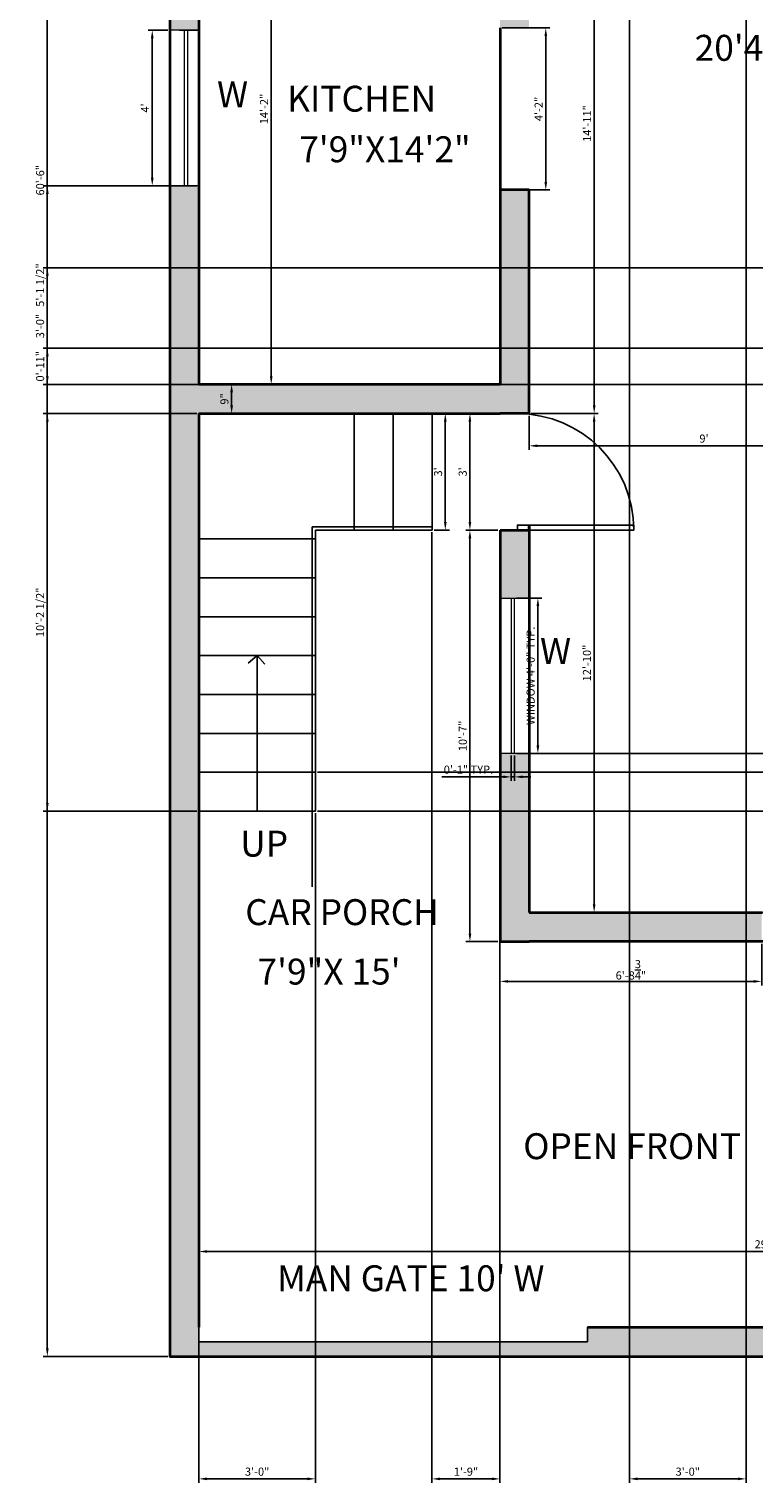
# Model space of a CAD drawing. Units: inches. Extents: x 844 to 1293, y 1224 to 2014.
# Tile 1 of 4: x 844 to 1068, y 1224 to 1673. Entities that reach past the tile are written whole.
import ezdxf

# ---------------------------------------------------------------- set-up
doc = ezdxf.new("R2010")
doc.units = ezdxf.units.IN
for name, color, linetype, lineweight in [('A-ANNO-DIMS', 2, 'Continuous', 18), ('A-ANNO-TEXT', 3, 'Continuous', 18), ('A-AREA-IDEN', 7, 'Continuous', 25), ('A-DOOR', 3, 'Continuous', 25), ('A-FLOR-STRS', 7, 'Continuous', 25), ('A-GLAZ', 4, 'Continuous', 18), ('A-WALL', 7, 'Continuous', 35), ('A-WALL-PATT', 252, 'Continuous', 13)]:
    doc.layers.add(name, color=color, linetype=linetype, lineweight=lineweight)
doc.styles.get("Standard").update_dxf_attribs({"font": 'arial.ttf'})
doc.dimstyles.new('Copy of ISO-25', dxfattribs={"dimtxt": 2.5, "dimasz": 2.5, "dimexe": 1.25, "dimexo": 0.625, "dimtad": 1, "dimlunit": 4, "dimtxsty": 'Standard', "dimcen": 2.5, "dimadec": 0, "dimazin": 0, "dimtfac": 1, "dimtmove": 0, "dimatfit": 3, "dimfxl": 1, "dimarcsym": 0})

# ---------------------------------------------------------------- blocks, each defined once
blk = doc.blocks.new('*U4')
for p, q in [((0, 0), (0, -6)), ((-40, 0), (-40, -6))]:
    blk.add_line(p, q)
blk.add_lwpolyline([(0, 0), (0, 40), (-1.75, 40), (-1.75, 0)], close=True)
blk.add_arc((0, 0), 40, 90, 180)
blk = doc.blocks.new('*D16')
at = {"layer": 'A-ANNO-DIMS', "color": 0, "lineweight": -2, "transparency": 16777216}
for p, q in [((897.09, 1733.04), (920.05, 1733.04)), ((918.8, 1730.54), (918.8, 1565.54)), ((897.09, 1563.04), (920.05, 1563.04))]:
    blk.add_line(p, q, dxfattribs=at)
at = {"layer": 'A-ANNO-DIMS', "color": 0, "transparency": 16777216}
for points in [[(918.39, 1730.54), (919.22, 1730.54), (918.8, 1733.04)], [(918.39, 1565.54), (919.22, 1565.54), (918.8, 1563.04)]]:
    blk.add_solid(points, dxfattribs=at)
at = {"layer": 'Defpoints', "color": 0, "transparency": 16777216}
for p in [(896.46, 1733.04), (896.46, 1563.04), (918.8, 1563.04)]:
    blk.add_point(p, dxfattribs=at)
at = {"layer": 'A-ANNO-DIMS', "color": 0, "transparency": 16777216, "insert": (916.92, 1648.04), "char_height": 2.5, "attachment_point": 5, "rotation": 90}
blk.add_mtext('14\'-2"', dxfattribs=at)
blk = doc.blocks.new('*D17')
at = {"layer": 'A-ANNO-DIMS', "color": 0, "lineweight": -2, "transparency": 16777216}
for p, q in [((998.46, 1553.35), (998.46, 1542.83)), ((1106.46, 1553.35), (1106.46, 1542.83)), ((1000.96, 1544.08), (1103.96, 1544.08))]:
    blk.add_line(p, q, dxfattribs=at)
at = {"layer": 'A-ANNO-DIMS', "color": 0, "transparency": 16777216}
for points in [[(1000.96, 1544.49), (1000.96, 1543.66), (998.46, 1544.08)], [(1103.96, 1544.49), (1103.96, 1543.66), (1106.46, 1544.08)]]:
    blk.add_solid(points, dxfattribs=at)
at = {"layer": 'Defpoints', "color": 0, "transparency": 16777216}
for p in [(998.46, 1553.98), (1106.46, 1553.98), (1106.46, 1544.08)]:
    blk.add_point(p, dxfattribs=at)
at = {"layer": 'A-ANNO-DIMS', "color": 0, "transparency": 16777216, "insert": (1052.46, 1545.98), "char_height": 2.5, "attachment_point": 5}
blk.add_mtext("9'", dxfattribs=at)
blk = doc.blocks.new('*D19')
at = {"layer": 'A-ANNO-DIMS', "color": 0, "lineweight": -2, "transparency": 16777216}
for p, q in [((999.09, 1733.04), (1019.81, 1733.04)), ((1018.56, 1730.54), (1018.56, 1556.54)), ((999.09, 1554.04), (1019.81, 1554.04))]:
    blk.add_line(p, q, dxfattribs=at)
at = {"layer": 'A-ANNO-DIMS', "color": 0, "transparency": 16777216}
for points in [[(1018.14, 1730.54), (1018.97, 1730.54), (1018.56, 1733.04)], [(1018.14, 1556.54), (1018.97, 1556.54), (1018.56, 1554.04)]]:
    blk.add_solid(points, dxfattribs=at)
at = {"layer": 'Defpoints', "color": 0, "transparency": 16777216}
for p in [(998.46, 1733.04), (998.46, 1554.04), (1018.56, 1554.04)]:
    blk.add_point(p, dxfattribs=at)
at = {"layer": 'A-ANNO-DIMS', "color": 0, "transparency": 16777216, "insert": (1016.68, 1643.54), "char_height": 2.5, "attachment_point": 5, "rotation": 90}
blk.add_mtext('14\'-11"', dxfattribs=at)
blk = doc.blocks.new('*D21')
at = {"layer": 'A-ANNO-DIMS', "color": 0, "lineweight": -2, "transparency": 16777216}
for p, q in [((989.46, 1390.05), (989.46, 1377.52)), ((1070.31, 1390.42), (1070.31, 1377.52)), ((991.96, 1378.77), (1067.81, 1378.77))]:
    blk.add_line(p, q, dxfattribs=at)
at = {"layer": 'A-ANNO-DIMS', "color": 0, "transparency": 16777216}
for points in [[(991.96, 1379.19), (991.96, 1378.36), (989.46, 1378.77)], [(1067.81, 1379.19), (1067.81, 1378.36), (1070.31, 1378.77)]]:
    blk.add_solid(points, dxfattribs=at)
at = {"layer": 'Defpoints', "color": 0, "transparency": 16777216}
for p in [(1070.31, 1391.04), (989.46, 1390.68), (1070.31, 1378.77)]:
    blk.add_point(p, dxfattribs=at)
at = {"layer": 'A-ANNO-DIMS', "color": 0, "transparency": 16777216, "insert": (1029.89, 1382.36), "char_height": 2.5, "attachment_point": 5}
blk.add_mtext('6\'-8{\\H1x;\\S3/4;}"', dxfattribs=at)
blk = doc.blocks.new('*D25')
at = {"layer": 'A-ANNO-DIMS', "color": 0, "lineweight": -2, "transparency": 16777216}
for p, q in [((988.84, 1518.04), (978.92, 1518.04)), ((980.17, 1393.54), (980.17, 1515.54)), ((988.84, 1391.04), (978.92, 1391.04))]:
    blk.add_line(p, q, dxfattribs=at)
at = {"layer": 'A-ANNO-DIMS', "color": 0, "transparency": 16777216}
for points in [[(979.76, 1515.54), (980.59, 1515.54), (980.17, 1518.04)], [(979.76, 1393.54), (980.59, 1393.54), (980.17, 1391.04)]]:
    blk.add_solid(points, dxfattribs=at)
at = {"layer": 'Defpoints', "color": 0, "transparency": 16777216}
for p in [(980.17, 1518.04), (989.46, 1518.04), (989.46, 1391.04)]:
    blk.add_point(p, dxfattribs=at)
at = {"layer": 'A-ANNO-DIMS', "color": 0, "transparency": 16777216, "insert": (978.27, 1454.54), "char_height": 2.5, "attachment_point": 5, "rotation": 90}
blk.add_mtext('10\'-7"', dxfattribs=at)
blk = doc.blocks.new('*D28')
at = {"layer": 'A-ANNO-DIMS', "color": 0, "lineweight": -2, "transparency": 16777216}
for p, q in [((988.84, 1554.04), (978.92, 1554.04)), ((980.17, 1520.54), (980.17, 1551.54)), ((988.84, 1518.04), (978.92, 1518.04))]:
    blk.add_line(p, q, dxfattribs=at)
at = {"layer": 'A-ANNO-DIMS', "color": 0, "transparency": 16777216}
for points in [[(979.75, 1551.54), (980.58, 1551.54), (980.17, 1554.04)], [(979.75, 1520.54), (980.58, 1520.54), (980.17, 1518.04)]]:
    blk.add_solid(points, dxfattribs=at)
at = {"layer": 'Defpoints', "color": 0, "transparency": 16777216}
for p in [(980.17, 1554.04), (989.46, 1554.04), (989.46, 1518.04)]:
    blk.add_point(p, dxfattribs=at)
at = {"layer": 'A-ANNO-DIMS', "color": 0, "transparency": 16777216, "insert": (978.27, 1536.04), "char_height": 2.5, "attachment_point": 5, "rotation": 90}
blk.add_mtext("3'", dxfattribs=at)
blk = doc.blocks.new('*D29')
at = {"layer": 'A-ANNO-DIMS', "color": 0, "lineweight": -2, "transparency": 16777216}
for p, q in [((999.09, 1554.04), (1019.79, 1554.04)), ((1018.54, 1402.54), (1018.54, 1551.54)), ((999.09, 1400.04), (1019.79, 1400.04))]:
    blk.add_line(p, q, dxfattribs=at)
at = {"layer": 'A-ANNO-DIMS', "color": 0, "transparency": 16777216}
for points in [[(1018.12, 1551.54), (1018.95, 1551.54), (1018.54, 1554.04)], [(1018.12, 1402.54), (1018.95, 1402.54), (1018.54, 1400.04)]]:
    blk.add_solid(points, dxfattribs=at)
at = {"layer": 'Defpoints', "color": 0, "transparency": 16777216}
for p in [(998.46, 1554.04), (1018.54, 1554.04), (998.46, 1400.04)]:
    blk.add_point(p, dxfattribs=at)
at = {"layer": 'A-ANNO-DIMS', "color": 0, "transparency": 16777216, "insert": (1016.64, 1477.04), "char_height": 2.5, "attachment_point": 5, "rotation": 90}
blk.add_mtext('12\'-10"', dxfattribs=at)
blk = doc.blocks.new('*D31')
at = {"layer": 'A-ANNO-DIMS', "color": 0, "lineweight": -2, "transparency": 16777216}
for p, q in [((896.46, 1272.67), (896.46, 1296.66)), ((1241.96, 1295.41), (898.96, 1295.41)), ((1244.46, 1272.67), (1244.46, 1296.66))]:
    blk.add_line(p, q, dxfattribs=at)
at = {"layer": 'A-ANNO-DIMS', "color": 0, "transparency": 16777216}
for points in [[(898.96, 1295.83), (898.96, 1295), (896.46, 1295.41)], [(1241.96, 1295.83), (1241.96, 1295), (1244.46, 1295.41)]]:
    blk.add_solid(points, dxfattribs=at)
at = {"layer": 'Defpoints', "color": 0, "transparency": 16777216}
for p in [(896.46, 1295.41), (896.46, 1272.04), (1244.46, 1272.04)]:
    blk.add_point(p, dxfattribs=at)
at = {"layer": 'A-ANNO-DIMS', "color": 0, "transparency": 16777216, "insert": (1070.46, 1297.32), "char_height": 2.5, "attachment_point": 5}
blk.add_mtext("29'", dxfattribs=at)
blk = doc.blocks.new('*D37')
at = {"layer": 'A-ANNO-DIMS', "color": 0, "lineweight": -2, "transparency": 16777216}
for p, q in [((897.09, 1563.04), (907.83, 1563.04)), ((906.58, 1560.54), (906.58, 1556.54)), ((897.09, 1554.04), (907.83, 1554.04))]:
    blk.add_line(p, q, dxfattribs=at)
at = {"layer": 'A-ANNO-DIMS', "color": 0, "transparency": 16777216}
for points in [[(906.16, 1560.54), (907, 1560.54), (906.58, 1563.04)], [(906.16, 1556.54), (907, 1556.54), (906.58, 1554.04)]]:
    blk.add_solid(points, dxfattribs=at)
at = {"layer": 'Defpoints', "color": 0, "transparency": 16777216}
for p in [(896.46, 1563.04), (896.46, 1554.04), (906.58, 1554.04)]:
    blk.add_point(p, dxfattribs=at)
at = {"layer": 'A-ANNO-DIMS', "color": 0, "transparency": 16777216, "insert": (904.68, 1558.54), "char_height": 2.5, "attachment_point": 5, "rotation": 90}
blk.add_mtext('9"', dxfattribs=at)
blk = doc.blocks.new('*D42')
at = {"layer": 'A-ANNO-DIMS', "color": 0, "lineweight": -2, "transparency": 16777216}
for p, q in [((990.09, 1673.04), (1004.85, 1673.04)), ((1003.6, 1625.54), (1003.6, 1670.54)), ((990.09, 1623.04), (1004.85, 1623.04))]:
    blk.add_line(p, q, dxfattribs=at)
at = {"layer": 'A-ANNO-DIMS', "color": 0, "transparency": 16777216}
for points in [[(1003.19, 1670.54), (1004.02, 1670.54), (1003.6, 1673.04)], [(1003.19, 1625.54), (1004.02, 1625.54), (1003.6, 1623.04)]]:
    blk.add_solid(points, dxfattribs=at)
at = {"layer": 'Defpoints', "color": 0, "transparency": 16777216}
for p in [(989.46, 1673.04), (1003.6, 1673.04), (989.46, 1623.04)]:
    blk.add_point(p, dxfattribs=at)
at = {"layer": 'A-ANNO-DIMS', "color": 0, "transparency": 16777216, "insert": (1001.72, 1648.04), "char_height": 2.5, "attachment_point": 5, "rotation": 90}
blk.add_mtext('4\'-2"', dxfattribs=at)
blk = doc.blocks.new('*D43')
at = {"layer": 'A-ANNO-DIMS', "color": 0, "lineweight": -2, "transparency": 16777216}
for p, q in [((886.84, 1672.34), (880.81, 1672.34)), ((882.06, 1626.84), (882.06, 1669.84)), ((886.84, 1624.34), (880.81, 1624.34))]:
    blk.add_line(p, q, dxfattribs=at)
at = {"layer": 'A-ANNO-DIMS', "color": 0, "transparency": 16777216}
for points in [[(881.64, 1669.84), (882.48, 1669.84), (882.06, 1672.34)], [(881.64, 1626.84), (882.48, 1626.84), (882.06, 1624.34)]]:
    blk.add_solid(points, dxfattribs=at)
at = {"layer": 'Defpoints', "color": 0, "transparency": 16777216}
for p in [(882.06, 1672.34), (887.46, 1672.34), (887.46, 1624.34)]:
    blk.add_point(p, dxfattribs=at)
at = {"layer": 'A-ANNO-DIMS', "color": 0, "transparency": 16777216, "insert": (880.18, 1648.34), "char_height": 2.5, "attachment_point": 5, "rotation": 90}
blk.add_mtext("4'", dxfattribs=at)
blk = doc.blocks.new('*D44')
at = {"layer": 'A-ANNO-DIMS', "color": 0, "lineweight": -2, "transparency": 16777216}
for p, q in [((969.09, 1554.04), (973.82, 1554.04)), ((972.57, 1551.54), (972.57, 1520.54)), ((969.09, 1518.04), (973.82, 1518.04))]:
    blk.add_line(p, q, dxfattribs=at)
at = {"layer": 'A-ANNO-DIMS', "color": 0, "transparency": 16777216}
for points in [[(972.15, 1551.54), (972.98, 1551.54), (972.57, 1554.04)], [(972.15, 1520.54), (972.98, 1520.54), (972.57, 1518.04)]]:
    blk.add_solid(points, dxfattribs=at)
at = {"layer": 'Defpoints', "color": 0, "transparency": 16777216}
for p in [(968.46, 1554.04), (968.46, 1518.04), (972.57, 1518.04)]:
    blk.add_point(p, dxfattribs=at)
at = {"layer": 'A-ANNO-DIMS', "color": 0, "transparency": 16777216, "insert": (970.67, 1536.04), "char_height": 2.5, "attachment_point": 5, "rotation": 90}
blk.add_mtext("3'", dxfattribs=at)
blk = doc.blocks.new('WIN-GLAZ-48IN')
for p, q in [((0, 48), (0, 0)), ((1, 48), (1, 0))]:
    blk.add_line(p, q)
blk = doc.blocks.new('*D49')
at = {"layer": 'A-ANNO-DIMS', "color": 0, "lineweight": -2, "transparency": 16777216}
for p, q in [((994.59, 1497.1), (1002.41, 1497.1)), ((1001.16, 1494.6), (1001.16, 1451.6)), ((994.59, 1449.1), (1002.41, 1449.1))]:
    blk.add_line(p, q, dxfattribs=at)
at = {"layer": 'A-ANNO-DIMS', "color": 0, "transparency": 16777216}
for points in [[(1000.75, 1494.6), (1001.58, 1494.6), (1001.16, 1497.1)], [(1000.75, 1451.6), (1001.58, 1451.6), (1001.16, 1449.1)]]:
    blk.add_solid(points, dxfattribs=at)
at = {"layer": 'Defpoints', "color": 0, "transparency": 16777216}
for p in [(993.96, 1497.1), (993.96, 1449.1), (1001.16, 1449.1)]:
    blk.add_point(p, dxfattribs=at)
at = {"layer": 'A-ANNO-DIMS', "color": 0, "transparency": 16777216, "insert": (999.25, 1473.1), "char_height": 2.5, "attachment_point": 5, "rotation": 90}
blk.add_mtext('WINDOW 4\'-0" TYP.', dxfattribs=at)
blk = doc.blocks.new('*D50')
at = {"layer": 'A-ANNO-DIMS', "color": 0, "lineweight": -2, "transparency": 16777216}
for p, q in [((992.96, 1448.48), (992.96, 1440.65)), ((993.96, 1448.48), (993.96, 1440.65)), ((990.46, 1441.9), (971.48, 1441.9)), ((993.96, 1441.9), (992.96, 1441.9)), ((996.46, 1441.9), (998.96, 1441.9))]:
    blk.add_line(p, q, dxfattribs=at)
at = {"layer": 'A-ANNO-DIMS', "color": 0, "transparency": 16777216}
for points in [[(990.46, 1442.32), (990.46, 1441.49), (992.96, 1441.9)], [(996.46, 1442.32), (996.46, 1441.49), (993.96, 1441.9)]]:
    blk.add_solid(points, dxfattribs=at)
at = {"layer": 'Defpoints', "color": 0, "transparency": 16777216}
for p in [(992.96, 1449.1), (993.96, 1449.1), (992.96, 1441.9)]:
    blk.add_point(p, dxfattribs=at)
at = {"layer": 'A-ANNO-DIMS', "color": 0, "transparency": 16777216, "insert": (979.72, 1443.81), "char_height": 2.5, "attachment_point": 5}
blk.add_mtext('0\'-1" TYP.', dxfattribs=at)
blk = doc.blocks.new('*D52')
at = {"layer": 'A-ANNO-DIMS', "color": 0, "lineweight": -2, "transparency": 16777216}
for p, q in [((886.84, 1989.04), (848.41, 1989.04)), ((849.66, 1265.54), (849.66, 1986.54)), ((886.84, 1263.04), (848.41, 1263.04))]:
    blk.add_line(p, q, dxfattribs=at)
at = {"layer": 'A-ANNO-DIMS', "color": 0, "transparency": 16777216}
for points in [[(849.25, 1986.54), (850.08, 1986.54), (849.66, 1989.04)], [(849.25, 1265.54), (850.08, 1265.54), (849.66, 1263.04)]]:
    blk.add_solid(points, dxfattribs=at)
at = {"layer": 'Defpoints', "color": 0, "transparency": 16777216}
for p in [(849.66, 1989.04), (887.46, 1989.04), (887.46, 1263.04)]:
    blk.add_point(p, dxfattribs=at)
at = {"layer": 'A-ANNO-DIMS', "color": 0, "transparency": 16777216, "insert": (847.76, 1626.04), "char_height": 2.5, "attachment_point": 5, "rotation": 90}
blk.add_mtext('60\'-6"', dxfattribs=at)
blk = doc.blocks.new('*D57')
at = {"layer": 'A-ANNO-DIMS', "color": 0, "lineweight": -2, "transparency": 16777216}
for p, q in [((895.84, 1624.34), (848.41, 1624.34)), ((849.66, 1565.54), (849.66, 1621.84)), ((895.84, 1563.04), (848.41, 1563.04))]:
    blk.add_line(p, q, dxfattribs=at)
at = {"layer": 'A-ANNO-DIMS', "color": 0, "transparency": 16777216}
for points in [[(849.25, 1621.84), (850.08, 1621.84), (849.66, 1624.34)], [(849.25, 1565.54), (850.08, 1565.54), (849.66, 1563.04)]]:
    blk.add_solid(points, dxfattribs=at)
at = {"layer": 'Defpoints', "color": 0, "transparency": 16777216}
for p in [(849.66, 1624.34), (896.46, 1624.34), (896.46, 1563.04)]:
    blk.add_point(p, dxfattribs=at)
at = {"layer": 'A-ANNO-DIMS', "color": 0, "transparency": 16777216, "insert": (847.75, 1593.69), "char_height": 2.5, "attachment_point": 5, "rotation": 90}
blk.add_mtext('5\'-1 1/2"', dxfattribs=at)
blk = doc.blocks.new('*D60')
at = {"layer": 'A-ANNO-DIMS', "color": 0, "lineweight": -2, "transparency": 16777216}
for p, q in [((1243.84, 1574.21), (848.41, 1574.21)), ((849.66, 1571.71), (849.66, 1565.54)), ((1243.84, 1563.04), (848.41, 1563.04))]:
    blk.add_line(p, q, dxfattribs=at)
at = {"layer": 'A-ANNO-DIMS', "color": 0, "transparency": 16777216}
for points in [[(849.25, 1571.71), (850.08, 1571.71), (849.66, 1574.21)], [(849.25, 1565.54), (850.08, 1565.54), (849.66, 1563.04)]]:
    blk.add_solid(points, dxfattribs=at)
at = {"layer": 'Defpoints', "color": 0, "transparency": 16777216}
for p in [(1244.46, 1574.21), (849.66, 1563.04), (1244.46, 1563.04)]:
    blk.add_point(p, dxfattribs=at)
at = {"layer": 'A-ANNO-DIMS', "color": 0, "transparency": 16777216, "insert": (847.76, 1568.63), "char_height": 2.5, "attachment_point": 5, "rotation": 90}
blk.add_mtext('0\'-11"', dxfattribs=at)
blk = doc.blocks.new('*D61')
at = {"layer": 'A-ANNO-DIMS', "color": 0, "lineweight": -2, "transparency": 16777216}
for p, q in [((999.09, 1449.1), (1292.51, 1449.1)), ((1291.26, 1402.54), (1291.26, 1446.6)), ((999.09, 1400.04), (1292.51, 1400.04))]:
    blk.add_line(p, q, dxfattribs=at)
at = {"layer": 'A-ANNO-DIMS', "color": 0, "transparency": 16777216}
for points in [[(1290.85, 1446.6), (1291.68, 1446.6), (1291.26, 1449.1)], [(1290.85, 1402.54), (1291.68, 1402.54), (1291.26, 1400.04)]]:
    blk.add_solid(points, dxfattribs=at)
at = {"layer": 'Defpoints', "color": 0, "transparency": 16777216}
for p in [(998.46, 1449.1), (1291.26, 1449.1), (998.46, 1400.04)]:
    blk.add_point(p, dxfattribs=at)
at = {"layer": 'A-ANNO-DIMS', "color": 0, "transparency": 16777216, "insert": (1289.38, 1424.57), "char_height": 2.5, "attachment_point": 5, "rotation": 90}
blk.add_mtext('4\'-1"', dxfattribs=at)
blk = doc.blocks.new('*D66')
at = {"layer": 'A-ANNO-DIMS', "color": 0, "lineweight": -2, "transparency": 16777216}
for p, q in [((1029.46, 1732.42), (1029.46, 1223.99)), ((1065.46, 1732.42), (1065.46, 1223.99)), ((1031.96, 1225.24), (1062.96, 1225.24))]:
    blk.add_line(p, q, dxfattribs=at)
at = {"layer": 'A-ANNO-DIMS', "color": 0, "transparency": 16777216}
for points in [[(1031.96, 1225.66), (1031.96, 1224.82), (1029.46, 1225.24)], [(1062.96, 1225.66), (1062.96, 1224.82), (1065.46, 1225.24)]]:
    blk.add_solid(points, dxfattribs=at)
at = {"layer": 'Defpoints', "color": 0, "transparency": 16777216}
for p in [(1029.46, 1733.04), (1065.46, 1733.04), (1065.46, 1225.24)]:
    blk.add_point(p, dxfattribs=at)
at = {"layer": 'A-ANNO-DIMS', "color": 0, "transparency": 16777216, "insert": (1047.46, 1227.14), "char_height": 2.5, "attachment_point": 5}
blk.add_mtext('3\'-0"', dxfattribs=at)
blk = doc.blocks.new('*D68')
at = {"layer": 'A-ANNO-DIMS', "color": 0, "lineweight": -2, "transparency": 16777216}
for p, q in [((1148.84, 1599.04), (848.41, 1599.04)), ((849.66, 1565.54), (849.66, 1596.54)), ((1148.84, 1563.04), (848.41, 1563.04))]:
    blk.add_line(p, q, dxfattribs=at)
at = {"layer": 'A-ANNO-DIMS', "color": 0, "transparency": 16777216}
for points in [[(849.25, 1596.54), (850.08, 1596.54), (849.66, 1599.04)], [(849.25, 1565.54), (850.08, 1565.54), (849.66, 1563.04)]]:
    blk.add_solid(points, dxfattribs=at)
at = {"layer": 'Defpoints', "color": 0, "transparency": 16777216}
for p in [(849.66, 1599.04), (1149.46, 1599.04), (1149.46, 1563.04)]:
    blk.add_point(p, dxfattribs=at)
at = {"layer": 'A-ANNO-DIMS', "color": 0, "transparency": 16777216, "insert": (847.76, 1581.04), "char_height": 2.5, "attachment_point": 5, "rotation": 90}
blk.add_mtext('3\'-0"', dxfattribs=at)
blk = doc.blocks.new('*D69')
at = {"layer": 'A-ANNO-DIMS', "color": 0, "lineweight": -2, "transparency": 16777216}
for p, q in [((896.46, 1430.7), (896.46, 1223.99)), ((932.46, 1430.7), (932.46, 1223.99)), ((898.96, 1225.24), (929.96, 1225.24))]:
    blk.add_line(p, q, dxfattribs=at)
at = {"layer": 'A-ANNO-DIMS', "color": 0, "transparency": 16777216}
for points in [[(898.96, 1225.66), (898.96, 1224.82), (896.46, 1225.24)], [(929.96, 1225.66), (929.96, 1224.82), (932.46, 1225.24)]]:
    blk.add_solid(points, dxfattribs=at)
at = {"layer": 'Defpoints', "color": 0, "transparency": 16777216}
for p in [(896.46, 1431.33), (932.46, 1431.33), (932.46, 1225.24)]:
    blk.add_point(p, dxfattribs=at)
at = {"layer": 'A-ANNO-DIMS', "color": 0, "transparency": 16777216, "insert": (914.46, 1227.14), "char_height": 2.5, "attachment_point": 5}
blk.add_mtext('3\'-0"', dxfattribs=at)
blk = doc.blocks.new('*D70')
at = {"layer": 'A-ANNO-DIMS', "color": 0, "lineweight": -2, "transparency": 16777216}
for p, q in [((895.84, 1554.04), (848.41, 1554.04)), ((849.66, 1433.83), (849.66, 1551.54)), ((895.84, 1431.33), (848.41, 1431.33))]:
    blk.add_line(p, q, dxfattribs=at)
at = {"layer": 'A-ANNO-DIMS', "color": 0, "transparency": 16777216}
for points in [[(849.25, 1551.54), (850.08, 1551.54), (849.66, 1554.04)], [(849.25, 1433.83), (850.08, 1433.83), (849.66, 1431.33)]]:
    blk.add_solid(points, dxfattribs=at)
at = {"layer": 'Defpoints', "color": 0, "transparency": 16777216}
for p in [(849.66, 1554.04), (896.46, 1554.04), (896.46, 1431.33)]:
    blk.add_point(p, dxfattribs=at)
at = {"layer": 'A-ANNO-DIMS', "color": 0, "transparency": 16777216, "insert": (847.75, 1492.68), "char_height": 2.5, "attachment_point": 5, "rotation": 90}
blk.add_mtext('10\'-2 1/2"', dxfattribs=at)
blk = doc.blocks.new('*D71')
at = {"layer": 'A-ANNO-DIMS', "color": 0, "lineweight": -2, "transparency": 16777216}
for p, q in [((933.09, 1443.33), (1292.51, 1443.33)), ((1291.26, 1433.83), (1291.26, 1440.83)), ((933.09, 1431.33), (1292.51, 1431.33))]:
    blk.add_line(p, q, dxfattribs=at)
at = {"layer": 'A-ANNO-DIMS', "color": 0, "transparency": 16777216}
for points in [[(1290.85, 1440.83), (1291.68, 1440.83), (1291.26, 1443.33)], [(1290.85, 1433.83), (1291.68, 1433.83), (1291.26, 1431.33)]]:
    blk.add_solid(points, dxfattribs=at)
at = {"layer": 'Defpoints', "color": 0, "transparency": 16777216}
for p in [(932.46, 1443.33), (1291.26, 1443.33), (932.46, 1431.33)]:
    blk.add_point(p, dxfattribs=at)
at = {"layer": 'A-ANNO-DIMS', "color": 0, "transparency": 16777216, "insert": (1289.36, 1437.33), "char_height": 2.5, "attachment_point": 5, "rotation": 90}
blk.add_mtext('1\'-0"', dxfattribs=at)
blk = doc.blocks.new('*D72')
at = {"layer": 'A-ANNO-DIMS', "color": 0, "lineweight": -2, "transparency": 16777216}
for p, q in [((968.46, 1517.42), (968.46, 1223.99)), ((989.46, 1517.42), (989.46, 1223.99)), ((970.96, 1225.24), (986.96, 1225.24))]:
    blk.add_line(p, q, dxfattribs=at)
at = {"layer": 'A-ANNO-DIMS', "color": 0, "transparency": 16777216}
for points in [[(970.96, 1225.66), (970.96, 1224.82), (968.46, 1225.24)], [(986.96, 1225.66), (986.96, 1224.82), (989.46, 1225.24)]]:
    blk.add_solid(points, dxfattribs=at)
at = {"layer": 'Defpoints', "color": 0, "transparency": 16777216}
for p in [(968.46, 1518.04), (989.46, 1518.04), (989.46, 1225.24)]:
    blk.add_point(p, dxfattribs=at)
at = {"layer": 'A-ANNO-DIMS', "color": 0, "transparency": 16777216, "insert": (978.96, 1227.14), "char_height": 2.5, "attachment_point": 5}
blk.add_mtext('1\'-9"', dxfattribs=at)

msp = doc.modelspace()

# ---------------------------------------------------------------- hatches: boundary and pattern name
at = {"layer": 'A-WALL-PATT'}
h = msp.add_hatch(color=256, dxfattribs=at)
h.dxf.hatch_style = 1
h.paths.add_polyline_path([(1253.465, 1989.042), (887.465, 1989.042), (887.465, 1920.042), (887.465, 1911.042), (887.465, 1871.621), (896.465, 1871.621), (896.465, 1911.042), (896.465, 1920.042), (896.465, 1980.042), (1000.465, 1980.042), (1244.465, 1980.042), (1244.465, 1968.042), (1253.465, 1968.042)])
h.paths.add_polyline_path([(1006.465, 1944.042), (1000.465, 1944.042), (1000.465, 1920.042), (896.465, 1920.042), (896.465, 1911.042), (1006.465, 1911.042), (1006.465, 1920.042)], flags=17)
h.paths.add_polyline_path([(1253.465, 1968.042), (1244.465, 1968.042), (1244.465, 1932.042), (1253.465, 1932.042)], flags=17)
h.paths.add_polyline_path([(1253.465, 1920.042), (1253.465, 1932.042), (1244.465, 1932.042), (1244.465, 1920.042), (1244.465, 1911.042), (1244.465, 1884.775), (1253.465, 1884.775), (1253.465, 1911.042)], flags=17)
h.paths.add_polyline_path([(1208.465, 1920.042), (1156.465, 1920.042), (1156.465, 1980.042), (1150.465, 1980.042), (1150.465, 1920.042), (1150.465, 1911.042), (1208.465, 1911.042)], flags=17)
h.paths.add_polyline_path([(1110.465, 1920.042), (1074.465, 1920.042), (1074.465, 1911.042), (1110.465, 1911.042)], flags=17)
h.paths.add_polyline_path([(896.465, 1811.621), (887.465, 1811.621), (887.465, 1672.343), (896.465, 1672.343), (896.465, 1733.042), (896.465, 1742.042)])
h.paths.add_polyline_path([(896.465, 1624.343), (887.465, 1624.343), (887.465, 1263.042), (1253.465, 1263.042), (1253.465, 1574.212), (1244.465, 1574.212), (1244.465, 1563.042), (1244.465, 1554.042), (1244.465, 1272.042), (1016.465, 1272.042), (1016.465, 1267.542), (896.465, 1267.542), (896.465, 1272.042), (896.465, 1554.042), (968.465, 1554.042), (989.465, 1554.042), (998.465, 1554.042), (998.465, 1623.042), (989.465, 1623.042), (989.465, 1563.042), (896.465, 1563.042)])
h.paths.add_polyline_path([(998.465, 1518.042), (994.855, 1518.042), (989.465, 1518.042), (989.465, 1497.104), (998.465, 1497.104)], flags=17)
h.paths.add_polyline_path([(998.465, 1449.104), (989.465, 1449.104), (989.465, 1391.042), (998.465, 1391.042), (1070.313, 1391.042), (1070.313, 1396.464), (1070.313, 1400.042), (998.465, 1400.042)], flags=17)
h.paths.add_polyline_path([(1112.465, 1450.531), (1106.465, 1450.531), (1106.465, 1400.042), (1106.465, 1391.042), (1112.465, 1391.042)], flags=17)
h.paths.add_polyline_path([(1112.465, 1554.042), (1112.394, 1554.042), (1112.394, 1559.602, -0.015479), (1112.465, 1561.896), (1112.465, 1563.042), (1106.465, 1563.042), (1106.465, 1554.042), (1106.465, 1510.531), (1112.465, 1510.531)], flags=17)
h.paths.add_polyline_path([(1158.465, 1623.042), (1244.465, 1623.042), (1244.465, 1632.042), (1158.465, 1632.042), (1149.465, 1632.042), (1149.465, 1599.042), (1158.465, 1599.042)])
h.paths.add_polyline_path([(1244.465, 1563.042), (1158.465, 1563.042), (1149.465, 1563.042), (1149.465, 1554.042), (1244.465, 1554.042)], flags=17)
h.paths.add_polyline_path([(1253.465, 1650.728), (1244.465, 1650.728), (1244.465, 1610.212), (1253.465, 1610.212)])
h.paths.add_polyline_path([(998.465, 1733.042), (989.465, 1733.042), (989.465, 1673.042), (998.465, 1673.042)])
h.paths.add_polyline_path([(1029.465, 1742.042), (896.465, 1742.042), (896.465, 1733.042), (989.465, 1733.042), (1029.465, 1733.042)])
h.paths.add_polyline_path([(1244.465, 1742.042), (1110.465, 1742.042), (1110.465, 1739.692, -0.0113533), (1110.5, 1738.147), (1110.5, 1733.042), (1244.465, 1733.042)])
h.paths.add_polyline_path([(1253.465, 1812.775), (1244.465, 1812.775), (1244.465, 1710.728), (1253.465, 1710.728)])
h.paths.add_polyline_path([(1074.465, 1911.042), (1074.465, 1920.042), (1065.465, 1920.042), (1065.465, 1911.042), (1065.465, 1742.042), (1065.465, 1733.042), (1074.465, 1733.042), (1074.465, 1742.042)])
h.paths.add_polyline_path([(1067.758, 1736.261), (1072.19, 1736.261), (1072.19, 1741.413), (1067.758, 1741.413)], flags=24)
h.paths.add_polyline_path([(975.783, 1886.472), (985.93, 1886.472), (985.93, 1891.624), (975.783, 1891.624)], flags=25)
h.paths.add_polyline_path([(917.205, 1821.36), (917.205, 1831.507), (912.053, 1831.507), (912.053, 1821.36)], flags=9)
h.paths.add_polyline_path([(1050.545, 1543.381), (1054.404, 1543.381), (1054.404, 1548.533), (1050.545, 1548.533)], flags=25)
h.paths.add_polyline_path([(1116.422, 1711.778), (1126.569, 1711.778), (1126.569, 1716.93), (1116.422, 1716.93)], flags=9)
h.paths.add_polyline_path([(1019.298, 1637.389), (1019.298, 1649.478), (1014.146, 1649.478), (1014.146, 1637.389)], flags=9)
h.paths.add_polyline_path([(980.864, 1534.121), (980.864, 1537.98), (975.712, 1537.98), (975.712, 1534.121)], flags=25)
h.paths.add_polyline_path([(1019.234, 1470.889), (1019.234, 1482.978), (1014.082, 1482.978), (1014.082, 1470.889)], flags=25)
h.paths.add_polyline_path([(1175.456, 1538.714), (1181.257, 1538.714), (1181.257, 1543.865), (1175.456, 1543.865)], flags=25)
h.paths.add_polyline_path([(1122.736, 1467.36), (1122.736, 1477.507), (1117.584, 1477.507), (1117.584, 1467.36)], flags=25)
h.paths.add_polyline_path([(907.276, 1556.335), (907.276, 1560.767), (902.124, 1560.767), (902.124, 1556.335)], flags=24)
h.paths.add_polyline_path([(1107.309, 1567.013), (1111.742, 1567.013), (1111.742, 1572.165), (1107.309, 1572.165)], flags=25)
h.paths.add_polyline_path([(955.783, 1784.038), (965.93, 1784.038), (965.93, 1789.19), (955.783, 1789.19)], flags=9)
h.paths.add_polyline_path([(1004.344, 1643.999), (1004.344, 1652.203), (999.192, 1652.203), (999.192, 1643.999)], flags=9)
h.paths.add_polyline_path([(973.263, 1534.121), (973.263, 1537.98), (968.111, 1537.98), (968.111, 1534.121)], flags=25)
h.paths.add_polyline_path([(1047.536, 1660.728), (1114.78, 1660.728), (1114.78, 1672.982), (1047.536, 1672.982)], flags=9)
h.paths.add_polyline_path([(1047.509, 1673.552), (1128.636, 1673.552), (1128.636, 1685.969), (1047.509, 1685.969)], flags=9)
h.paths.add_polyline_path([(999.825, 1474.75), (1014.374, 1474.75), (1014.374, 1486.75), (999.825, 1486.75)], flags=25)
h.paths.add_polyline_path([(1085.974, 1473.689), (1100.523, 1473.689), (1100.523, 1485.689), (1085.974, 1485.689)], flags=25)
h.paths.add_polyline_path([(898.914, 1844.786), (913.462, 1844.786), (913.462, 1856.786), (898.914, 1856.786)], flags=9)
h.paths.add_polyline_path([(1021.801, 1899.15), (1036.35, 1899.15), (1036.35, 1911.15), (1021.801, 1911.15)], flags=25)
h.paths.add_polyline_path([(933.371, 1817.465), (997.445, 1817.465), (997.445, 1829.522), (933.371, 1829.522)], flags=9)
h.paths.add_polyline_path([(912.536, 1375.627), (960.277, 1375.627), (960.277, 1387.881), (912.536, 1387.881)], flags=25)
h.paths.add_polyline_path([(908.723, 1393.944), (979.923, 1393.944), (979.923, 1406.361), (908.723, 1406.361)], flags=25)
h.paths.add_polyline_path([(907.199, 1415.111), (926.792, 1415.111), (926.792, 1427.316), (907.199, 1427.316)], flags=25)
h.paths.add_polyline_path([(1130.034, 1467.266), (1180.017, 1467.266), (1180.017, 1479.52), (1130.034, 1479.52)], flags=25)
h.paths.add_polyline_path([(1130.007, 1480.09), (1210.517, 1480.09), (1210.517, 1492.508), (1130.007, 1492.508)], flags=25)
h.paths.add_polyline_path([(918.552, 1280.947), (1012.38, 1280.947), (1012.38, 1293.356), (918.552, 1293.356)], flags=25)
h.paths.add_polyline_path([(1074.912, 1322.783), (1119.613, 1322.783), (1119.613, 1334.988), (1074.912, 1334.988)], flags=25)
h.paths.add_polyline_path([(994.568, 1321.709), (1075.078, 1321.709), (1075.078, 1334.127), (994.568, 1334.127)], flags=25)
h.paths.add_polyline_path([(932.502, 1835.432), (1188.778, 1835.432), (1188.778, 1847.849), (932.502, 1847.849)], flags=9)

# ---------------------------------------------------------------- linework, layer by layer
at = {"layer": 'A-DOOR'}
for p, q in [((896.465, 1272.042), (896.465, 1267.542)), ((1016.465, 1267.542), (1016.465, 1272.042)), ((1016.465, 1267.542), (896.465, 1267.542)), ((1016.465, 1267.542), (1016.465, 1267.542)), ((896.465, 1263.042), (1016.465, 1263.042))]:
    msp.add_line(p, q, dxfattribs=at)
at = {"layer": 'A-FLOR-STRS'}
for p, q in [((896.465, 1554.042), (968.465, 1554.042)), ((944.465, 1518.042), (944.465, 1554.042)), ((944.465, 1554.042), (956.465, 1554.042)), ((989.465, 1554.042), (953.465, 1554.042)), ((956.465, 1554.042), (956.465, 1518.042)), ((968.465, 1554.042), (968.465, 1518.042)), ((932.465, 1519.042), (931.465, 1519.042)), ((931.465, 1519.042), (931.465, 1431.328)), ((968.465, 1519.042), (932.465, 1519.042)), ((968.465, 1518.042), (932.465, 1518.042)), ((932.465, 1518.042), (932.465, 1431.328)), ((932.465, 1518.042), (944.465, 1518.042)), ((968.465, 1518.042), (968.465, 1519.042)), ((896.465, 1503.328), (896.465, 1515.328)), ((896.465, 1515.328), (932.465, 1515.328)), ((932.465, 1503.328), (896.465, 1503.328)), ((932.465, 1491.328), (932.465, 1503.328)), ((896.465, 1479.328), (896.465, 1491.328)), ((896.465, 1491.328), (932.465, 1491.328)), ((932.465, 1479.328), (896.465, 1479.328)), ((914.465, 1479.328), (911.732, 1476.945)), ((914.465, 1431.328), (914.465, 1479.328)), ((914.465, 1479.328), (916.785, 1476.668)), ((932.465, 1467.328), (932.465, 1479.328)), ((896.465, 1455.328), (896.465, 1467.328)), ((896.465, 1467.328), (932.465, 1467.328)), ((932.465, 1455.328), (896.465, 1455.328)), ((932.465, 1443.328), (932.465, 1455.328)), ((896.465, 1431.328), (896.465, 1443.328)), ((896.465, 1443.328), (932.465, 1443.328)), ((932.465, 1431.328), (896.465, 1431.328)), ((931.465, 1431.328), (931.465, 1408.011))]:
    msp.add_line(p, q, dxfattribs=at)
at = {"layer": 'A-GLAZ'}
for p, q in [((896.465, 1672.343), (887.465, 1672.343)), ((890.465, 1672.343), (896.465, 1672.343)), ((896.465, 1672.343), (896.465, 1624.343)), ((896.465, 1624.343), (887.465, 1624.343)), ((896.465, 1624.343), (890.465, 1624.343)), ((989.465, 1497.104), (998.465, 1497.104)), ((998.465, 1497.104), (998.465, 1449.104)), ((998.465, 1449.104), (989.465, 1449.104))]:
    msp.add_line(p, q, dxfattribs=at)
at = {"layer": 'A-WALL'}
for p, q in [((896.465, 1733.042), (896.465, 1672.343)), ((989.465, 1673.042), (989.465, 1623.042)), ((998.465, 1623.042), (989.465, 1623.042)), ((989.465, 1623.042), (989.465, 1563.042)), ((998.465, 1554.042), (998.465, 1623.042)), ((989.465, 1563.042), (896.465, 1563.042)), ((896.465, 1554.042), (989.465, 1554.042)), ((998.465, 1554.042), (989.465, 1554.042)), ((998.465, 1554.042), (998.465, 1553.977)), ((998.465, 1553.977), (998.465, 1554.042)), ((989.465, 1518.042), (989.465, 1391.042)), ((989.465, 1518.042), (998.465, 1518.042)), ((989.465, 1518.042), (989.465, 1497.104)), ((998.465, 1518.042), (998.465, 1519.614)), ((998.465, 1519.614), (998.465, 1400.042)), ((998.465, 1400.042), (1070.465, 1400.042)), ((989.465, 1391.042), (998.465, 1391.042)), ((1112.465, 1391.042), (998.465, 1391.042))]:
    msp.add_line(p, q, dxfattribs=at)
for points in [[(887.465, 1911.042), (887.465, 1263.042), (1253.465, 1263.042), (1253.465, 1911.042)], [(896.465, 1911.042), (896.465, 1563.042)], [(1016.465, 1272.042), (1244.465, 1272.042), (1244.465, 1911.042)], [(896.465, 1554.042), (896.465, 1272.042)]]:
    msp.add_lwpolyline(points, dxfattribs=at)

# ---------------------------------------------------------------- block references
at = {"layer": 'A-DOOR', "xscale": 0.898373054501015, "yscale": 0.898373054501015, "zscale": 0.898373054501015, "rotation": 270}
msp.add_blockref('*U4', (994.855, 1518.042), dxfattribs=at)
at = {"layer": 'A-GLAZ'}
msp.add_blockref('WIN-GLAZ-48IN', (891.965, 1624.343), dxfattribs=at)
at = {"layer": 'A-GLAZ', "rotation": 180}
msp.add_blockref('WIN-GLAZ-48IN', (993.965, 1497.104), dxfattribs=at)

# ---------------------------------------------------------------- texts
at = {"layer": 'A-ANNO-TEXT'}
for s, p in [('W', (902.082, 1648.574)), ('W', (1001.825, 1476.75)), ('UP', (909.233, 1417.282)), ("MAN GATE 10' W", (920.62, 1283.152))]:
    msp.add_text(s, height=8, dxfattribs=at).set_placement(p)
at = {"layer": 'A-AREA-IDEN'}
for s, p in [('20\'4" X 14\'2"', (1049.578, 1662.907)), ('KITCHEN', (923.729, 1647.203)), ('7\'9"X14\'2"', (927.456, 1631.598)), ('CAR PORCH', (910.792, 1396.15)), ('7\'9"X 15\'', (914.578, 1377.806)), ('OPEN FRONT ', (996.637, 1323.915))]:
    msp.add_text(s, height=8, dxfattribs=at).set_placement(p)

# ---------------------------------------------------------------- dimensions: what is measured, and where the dimension line sits
at = {"layer": 'A-ANNO-DIMS'}
for base, p1, p2, override, picture, middle in [((849.665, 1989.042), (887.465, 1263.042), (887.465, 1989.042), {"dimdec": 1, "dimlfac": 1, "dimrnd": 0, "dimzin": 1, "dimdsep": 46, "dimlunit": 4, "dimfrac": 2}, '*D52', (847.763, 1626.042)), ((918.805, 1563.042), (896.465, 1733.042), (896.465, 1563.042), {"dimclrd": 0, "dimclre": 0, "dimclrt": 0}, '*D16', (916.925, 1648.042)), ((1018.558, 1554.042), (998.465, 1733.042), (998.465, 1554.042), {"dimclrd": 0, "dimclre": 0, "dimclrt": 0}, '*D19', (1016.678, 1643.542)), ((882.06, 1672.343), (887.465, 1624.343), (887.465, 1672.343), {"dimclrd": 0, "dimclre": 0, "dimclrt": 0}, '*D43', (880.185, 1648.343)), ((1003.604, 1673.042), (989.465, 1623.042), (989.465, 1673.042), {"dimclrd": 0, "dimclre": 0, "dimclrt": 0}, '*D42', (1001.724, 1648.042)), ((849.665, 1624.343), (896.465, 1563.042), (896.465, 1624.343), {"dimdec": 1, "dimlfac": 1, "dimrnd": 0, "dimzin": 1, "dimdsep": 46, "dimlunit": 4, "dimfrac": 2}, '*D57', (847.747, 1593.693)), ((849.665, 1599.042), (1149.465, 1563.042), (1149.465, 1599.042), {"dimdec": 1, "dimlfac": 1, "dimrnd": 0, "dimzin": 1, "dimdsep": 46, "dimlunit": 4, "dimfrac": 2}, '*D68', (847.763, 1581.042)), ((849.665, 1563.042), (1244.465, 1574.212), (1244.465, 1563.042), {"dimdec": 1, "dimlfac": 1, "dimrnd": 0, "dimzin": 1, "dimdsep": 46, "dimlunit": 4, "dimfrac": 2}, '*D60', (847.763, 1568.627)), ((906.578, 1554.042), (896.465, 1563.042), (896.465, 1554.042), {"dimclrd": 0, "dimclre": 0, "dimclrt": 0}, '*D37', (904.677, 1558.542)), ((849.665, 1554.042), (896.465, 1431.328), (896.465, 1554.042), {"dimdec": 1, "dimlfac": 1, "dimrnd": 0, "dimzin": 1, "dimdsep": 46, "dimlunit": 4, "dimfrac": 2}, '*D70', (847.747, 1492.685)), ((972.567, 1518.042), (968.465, 1554.042), (968.465, 1518.042), {"dimclrd": 0, "dimclre": 0, "dimclrt": 0}, '*D44', (970.665, 1536.042)), ((980.168, 1554.042), (989.465, 1518.042), (989.465, 1554.042), {"dimclrd": 0, "dimclre": 0, "dimclrt": 0}, '*D28', (978.266, 1536.042)), ((1018.537, 1554.042), (998.465, 1400.042), (998.465, 1554.042), {"dimclrd": 0, "dimclre": 0, "dimclrt": 0}, '*D29', (1016.635, 1477.042)), ((980.173, 1518.042), (989.465, 1391.042), (989.465, 1518.042), {"dimclrd": 0, "dimclre": 0, "dimclrt": 0}, '*D25', (978.271, 1454.542)), ((1291.265, 1449.104), (998.465, 1400.042), (998.465, 1449.104), {"dimdec": 1, "dimlfac": 1, "dimrnd": 0, "dimzin": 1, "dimdsep": 46, "dimlunit": 4, "dimfrac": 2}, '*D61', (1289.385, 1424.573)), ((1291.265, 1443.328), (932.465, 1431.328), (932.465, 1443.328), {"dimdec": 1, "dimlfac": 1, "dimrnd": 0, "dimzin": 1, "dimdsep": 46, "dimlunit": 4, "dimfrac": 2}, '*D71', (1289.363, 1437.328))]:
    dim = msp.add_linear_dim(base=base, p1=p1, p2=p2, angle=90, dimstyle='Copy of ISO-25', override=override, dxfattribs=at)
    dim.commit()
    dim.dimension.update_dxf_attribs({"geometry": picture, "text_midpoint": middle})
for base, p1, p2, override, picture, middle in [((1065.465, 1225.242), (1029.465, 1733.042), (1065.465, 1733.042), {"dimdec": 1, "dimlfac": 1, "dimrnd": 0, "dimzin": 1, "dimdsep": 46, "dimlunit": 4, "dimfrac": 2}, '*D66', (1047.465, 1227.144)), ((1106.465, 1544.078), (998.465, 1553.977), (1106.465, 1553.977), {"dimclrd": 0, "dimclre": 0, "dimclrt": 0}, '*D17', (1052.465, 1545.98)), ((989.465, 1225.242), (968.465, 1518.042), (989.465, 1518.042), {"dimdec": 1, "dimlfac": 1, "dimrnd": 0, "dimzin": 1, "dimdsep": 46, "dimlunit": 4, "dimfrac": 2}, '*D72', (978.965, 1227.143)), ((932.465, 1225.242), (896.465, 1431.328), (932.465, 1431.328), {"dimdec": 1, "dimlfac": 1, "dimrnd": 0, "dimzin": 1, "dimdsep": 46, "dimlunit": 4, "dimfrac": 2}, '*D69', (914.465, 1227.144)), ((1070.313, 1378.774), (989.465, 1390.677), (1070.313, 1391.042), {"dimclrd": 0, "dimclre": 0, "dimclrt": 0}, '*D21', (1029.889, 1382.364)), ((896.465, 1295.414), (1244.465, 1272.042), (896.465, 1272.042), {"dimclrd": 0, "dimclre": 0, "dimclrt": 0}, '*D31', (1070.465, 1297.315))]:
    dim = msp.add_linear_dim(base=base, p1=p1, p2=p2, dimstyle='Copy of ISO-25', override=override, dxfattribs=at)
    dim.commit()
    dim.dimension.update_dxf_attribs({"geometry": picture, "text_midpoint": middle})
for base, p1, p2, angle, text, picture, middle in [((1001.165, 1449.104), (993.965, 1497.104), (993.965, 1449.104), 270, 'WINDOW <> TYP.', '*D49', (999.246, 1473.104)), ((992.965, 1441.904), (993.965, 1449.104), (992.965, 1449.104), 180, '<> TYP.', '*D50', (979.72, 1443.806))]:
    dim = msp.add_linear_dim(base=base, p1=p1, p2=p2, angle=angle, text=text, dimstyle='Copy of ISO-25', override={"dimdec": 1, "dimlfac": 1, "dimrnd": 0, "dimzin": 1, "dimdsep": 46, "dimlunit": 4, "dimfrac": 2}, dxfattribs=at)
    dim.commit()
    dim.dimension.update_dxf_attribs({"geometry": picture, "text_midpoint": middle})

doc.saveas('drawing.dxf')
